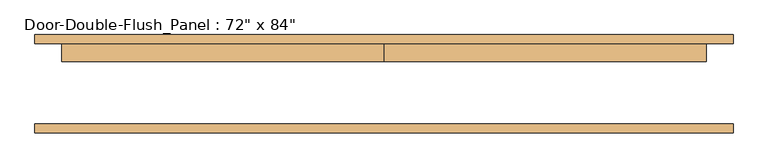
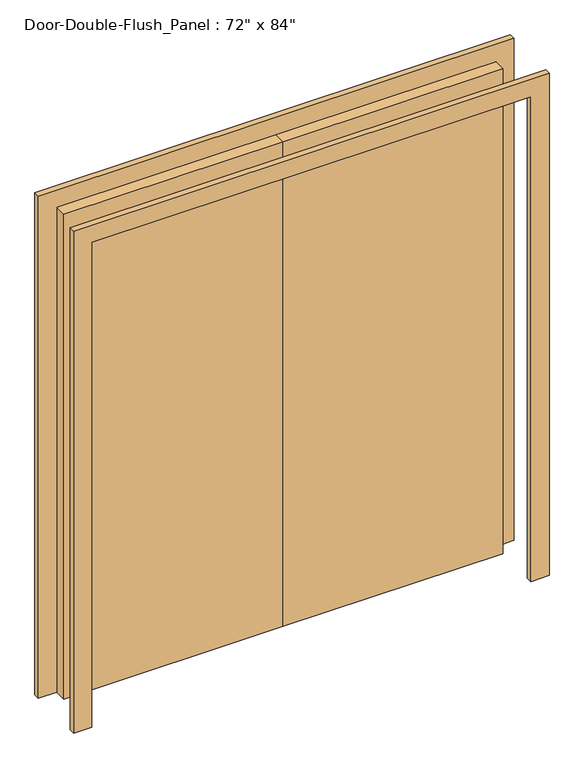
"""IFC4 building model written with IfcOpenShell, lengths in millimetres: door geometry."""

from ifc_helpers import new_model, si_unit, frame, origin, origin_with_axes, place, context, project, spatial, polyline, outline, extrude, source, transform, mapped, element, save


def door_640b4634(model_context):
    return source(origin(), model_context, "Body", "SweptSolid", [
        extrude(outline(polyline([(2133.6, -914.4), (2133.6, 914.4), (0.0, 914.4), (0.0, 990.6), (2209.8, 990.6), (2209.8, -990.6), (0.0, -990.6), (0.0, -914.4), (2133.6, -914.4)])), frame((0.0, -139.7, 0.0), z_axis=(0.0, 1.0, 0.0), x_axis=(0.0, 0.0, 1.0)), (0.0, 0.0, 1.0), 25.4),
        extrude(outline(polyline([(2133.6, -914.4), (2133.6, 914.4), (0.0, 914.4), (0.0, 990.6), (2209.8, 990.6), (2209.8, -990.6), (0.0, -990.6), (0.0, -914.4), (2133.6, -914.4)])), frame((0.0, 114.3, 0.0), z_axis=(0.0, 1.0, 0.0), x_axis=(0.0, 0.0, 1.0)), (0.0, 0.0, 1.0), 25.4),
        extrude(outline(polyline([(0.0, 114.3), (914.4, 114.3), (914.4, 63.5), (0.0, 63.5), (0.0, 114.3)])), origin_with_axes(), (0.0, 0.0, 1.0), 2133.6),
        extrude(outline(polyline([(-914.4, 114.3), (0.0, 114.3), (0.0, 63.5), (-914.4, 63.5), (-914.4, 114.3)])), origin_with_axes(), (0.0, 0.0, 1.0), 2133.6),
    ])


if __name__ == "__main__":
    model = new_model("IFC4")
    model_context = context("Model", 3, world=origin())
    ifc_project = project(units=[si_unit("LENGTHUNIT", "METRE", prefix="MILLI")], contexts=[model_context])
    site = spatial("IfcSite", under=ifc_project)
    building = spatial("IfcBuilding", under=site)
    placement = place(None, origin())
    door_shape = door_640b4634(model_context)
    element("IfcDoor", 1, ObjectType="Door-Double-Flush_Panel : 72\" x 84\"", at=placement, inside=building, context=model_context, shape_type="MappedRepresentation", body=[
        mapped(door_shape, transform((0.0, 0.0, 0.0), x_axis=(1.0, 0.0, 0.0), y_axis=(0.0, 1.0, 0.0), z_axis=(0.0, 0.0, 1.0))),
    ])
    save(model, "model.ifc")

# Revit data of these elements
# Type "Door-Double-Flush_Panel : 72\" x 84\""
#   Type Mark = "8"
#   Construction Type Id = "DOOR"
#   Assembly Code = "C1020"
#   Analytic Construction = "Wooden"
#   Thickness = 0' - 2"
#   Thermal Resistance (R) = 2.5876 (h·ft²·°F)/BTU
#   Swing Angle [instance default] = 90.00°
#   Panel Width = 3' - 0"
#   Heat Transfer Coefficient (U) = 0.3865 BTU/(h·ft²·°F)
#   Height = 7' - 0"
#   Trim Projection Ext = 0' - 1"
#   Trim Projection Int = 0' - 1"
#   Trim Width = 0' - 3"
#   Width = 6' - 0"
#   Define Thermal Properties by = 1
#   Panel Material = Wood - Birch - Solid Stained Light Low Gloss
#   Trim Material = Paint - Sienna
#   Visual Light Transmittance = 0
#   Solar Heat Gain Coefficient = 0
#   Function = (empty or 0)
#   Wall Closure = (empty or 0)
# Element 1 (IfcDoor, "Door-Double-Flush_Panel : 72\" x 84\"")
#   Materials on its faces: "Paint - Sienna", "Wood - Birch - Solid Stained Light Low Gloss"
# Materials
#   "Wood - Birch - Solid Stained Light Low Gloss": class "Wood", colour RGB 210 159 95, transparency 0, Cost = 0
#   "Paint - Sienna": colour RGB 118 70 51, transparency 0, Cost = 0
